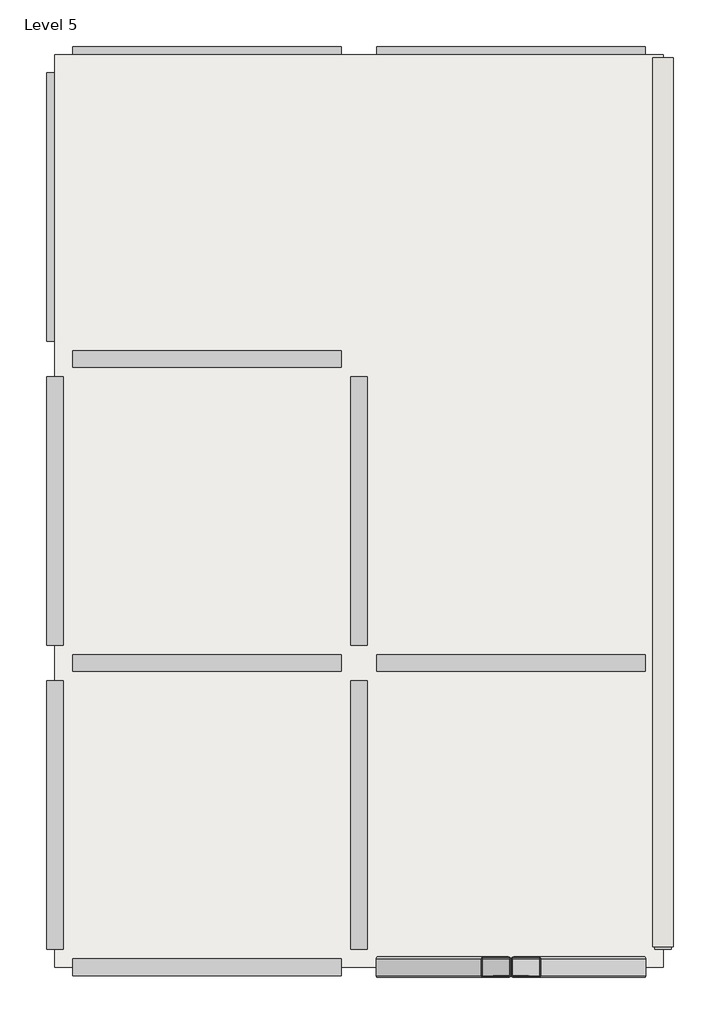
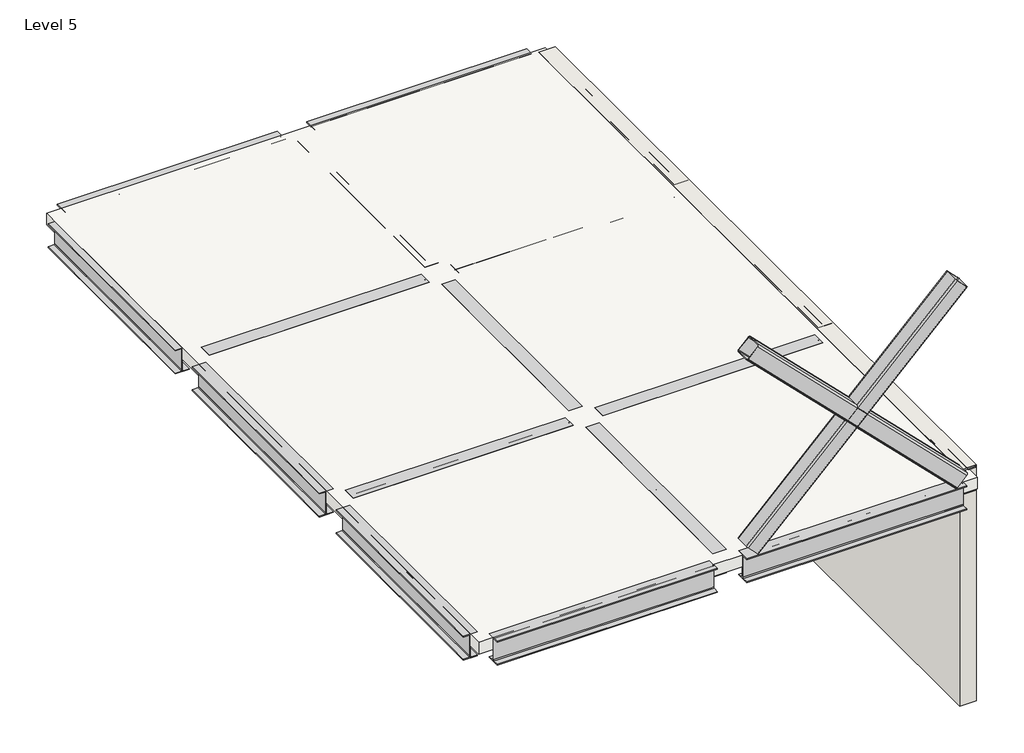
# One storey: 17 beams, 2 members, 1 slab, 1 wall.
"""IFC4 building model written with IfcOpenShell, lengths in millimetres."""

from ifc_helpers import new_model, si_unit, frame, origin, place, context, project, spatial, polyline, outline, extrude, transform, mapped, element, save
from components import ub_universal_beams_ub305x165x40_60ab2ee1, m_hss_square_hss203_2x203_2x9_5_07d005dd

model = new_model("IFC4")

# Units and contexts
model_context = context("Model", 3, world=origin())
ifc_project = project(units=[si_unit("LENGTHUNIT", "METRE", prefix="MILLI")], contexts=[model_context])

# Site, building, storey
site = spatial("IfcSite", under=ifc_project)
building = spatial("IfcBuilding", under=site)
storey = spatial("IfcBuildingStorey", under=building, Name="Level 5", Elevation=12000.0)

# Beams
placement = place(None, origin())
ub_universal_beams_ub305x165x40_shape = ub_universal_beams_ub305x165x40_60ab2ee1(model_context)
element("IfcBeam", 1, ObjectType="UB-Universal Beams : UB305x165x40", at=placement, inside=storey, context=model_context, shape_type="MappedRepresentation", body=[
    mapped(ub_universal_beams_ub305x165x40_shape, transform((18435.1404262, -6314.7314166, 11848.3), x_axis=(-1.0, 0.0, 0.0), y_axis=(0.0, -1.0, 0.0), z_axis=(0.0, 0.0, 1.0))),
])
element("IfcBeam", 2, ObjectType="UB-Universal Beams : UB305x165x40", at=placement, inside=storey, context=model_context, shape_type="MappedRepresentation", body=[
    mapped(ub_universal_beams_ub305x165x40_shape, transform((15435.1404262, -6314.7314166, 11848.3), x_axis=(-1.0, 0.0, 0.0), y_axis=(0.0, -1.0, 0.0), z_axis=(0.0, 0.0, 1.0))),
])
element("IfcBeam", 3, ObjectType="UB-Universal Beams : UB305x165x40", at=placement, inside=storey, context=model_context, shape_type="MappedRepresentation", body=[
    mapped(ub_universal_beams_ub305x165x40_shape, transform((13935.1404262, -4814.7314166, 11848.3), x_axis=(0.0, 1.0, 0.0), y_axis=(-1.0, 0.0, 0.0), z_axis=(0.0, 0.0, 1.0))),
])
element("IfcBeam", 4, ObjectType="UB-Universal Beams : UB305x165x40", at=placement, inside=storey, context=model_context, shape_type="MappedRepresentation", body=[
    mapped(ub_universal_beams_ub305x165x40_shape, transform((13935.1404262, -1814.7314166, 11848.3), x_axis=(0.0, 1.0, 0.0), y_axis=(-1.0, 0.0, 0.0), z_axis=(0.0, 0.0, 1.0))),
])
element("IfcBeam", 5, ObjectType="UB-Universal Beams : UB305x165x40", at=placement, inside=storey, context=model_context, shape_type="MappedRepresentation", body=[
    mapped(ub_universal_beams_ub305x165x40_shape, transform((13935.1404262, 1185.2685834, 11848.3), x_axis=(0.0, 1.0, 0.0), y_axis=(-1.0, 0.0, 0.0), z_axis=(0.0, 0.0, 1.0))),
])
element("IfcBeam", 6, ObjectType="UB-Universal Beams : UB305x165x40", at=placement, inside=storey, context=model_context, shape_type="MappedRepresentation", body=[
    mapped(ub_universal_beams_ub305x165x40_shape, transform((18435.1404262, -3314.7314166, 11848.3), x_axis=(-1.0, 0.0, 0.0), y_axis=(0.0, -1.0, 0.0), z_axis=(0.0, 0.0, 1.0))),
])
element("IfcBeam", 7, ObjectType="UB-Universal Beams : UB305x165x40", at=placement, inside=storey, context=model_context, shape_type="MappedRepresentation", body=[
    mapped(ub_universal_beams_ub305x165x40_shape, transform((15435.1404262, -3314.7314166, 11848.3), x_axis=(-1.0, 0.0, 0.0), y_axis=(0.0, -1.0, 0.0), z_axis=(0.0, 0.0, 1.0))),
])
element("IfcBeam", 8, ObjectType="UB-Universal Beams : UB305x165x40", at=placement, inside=storey, context=model_context, shape_type="MappedRepresentation", body=[
    mapped(ub_universal_beams_ub305x165x40_shape, transform((18435.1404262, -314.7314166, 11848.3), x_axis=(-1.0, 0.0, 0.0), y_axis=(0.0, -1.0, 0.0), z_axis=(0.0, 0.0, 1.0))),
])
element("IfcBeam", 9, ObjectType="UB-Universal Beams : UB305x165x40", at=placement, inside=storey, context=model_context, shape_type="MappedRepresentation", body=[
    mapped(ub_universal_beams_ub305x165x40_shape, transform((15435.1404262, -314.7314166, 11848.3), x_axis=(-1.0, 0.0, 0.0), y_axis=(0.0, -1.0, 0.0), z_axis=(0.0, 0.0, 1.0))),
])
element("IfcBeam", 10, ObjectType="UB-Universal Beams : UB305x165x40", at=placement, inside=storey, context=model_context, shape_type="MappedRepresentation", body=[
    mapped(ub_universal_beams_ub305x165x40_shape, transform((18435.1404262, 2685.2685834, 11848.3), x_axis=(-1.0, 0.0, 0.0), y_axis=(0.0, -1.0, 0.0), z_axis=(0.0, 0.0, 1.0))),
])
element("IfcBeam", 11, ObjectType="UB-Universal Beams : UB305x165x40", at=placement, inside=storey, context=model_context, shape_type="MappedRepresentation", body=[
    mapped(ub_universal_beams_ub305x165x40_shape, transform((15435.1404262, 2685.2685834, 11848.3), x_axis=(-1.0, 0.0, 0.0), y_axis=(0.0, -1.0, 0.0), z_axis=(0.0, 0.0, 1.0))),
])
element("IfcBeam", 12, ObjectType="UB-Universal Beams : UB305x165x40", at=placement, inside=storey, context=model_context, shape_type="MappedRepresentation", body=[
    mapped(ub_universal_beams_ub305x165x40_shape, transform((16935.1404262, -4814.7314166, 11848.3), x_axis=(0.0, 1.0, 0.0), y_axis=(-1.0, 0.0, 0.0), z_axis=(0.0, 0.0, 1.0))),
])
element("IfcBeam", 13, ObjectType="UB-Universal Beams : UB305x165x40", at=placement, inside=storey, context=model_context, shape_type="MappedRepresentation", body=[
    mapped(ub_universal_beams_ub305x165x40_shape, transform((16935.1404262, -1814.7314166, 11848.3), x_axis=(0.0, 1.0, 0.0), y_axis=(-1.0, 0.0, 0.0), z_axis=(0.0, 0.0, 1.0))),
])
element("IfcBeam", 14, ObjectType="UB-Universal Beams : UB305x165x40", at=placement, inside=storey, context=model_context, shape_type="MappedRepresentation", body=[
    mapped(ub_universal_beams_ub305x165x40_shape, transform((16935.1404262, 1185.2685834, 11848.3), x_axis=(0.0, 1.0, 0.0), y_axis=(-1.0, 0.0, 0.0), z_axis=(0.0, 0.0, 1.0))),
])
element("IfcBeam", 15, ObjectType="UB-Universal Beams : UB305x165x40", at=placement, inside=storey, context=model_context, shape_type="MappedRepresentation", body=[
    mapped(ub_universal_beams_ub305x165x40_shape, transform((19935.1404262, -1814.7314166, 11848.3), x_axis=(0.0, 1.0, 0.0), y_axis=(-1.0, 0.0, 0.0), z_axis=(0.0, 0.0, 1.0))),
])
element("IfcBeam", 16, ObjectType="UB-Universal Beams : UB305x165x40", at=placement, inside=storey, context=model_context, shape_type="MappedRepresentation", body=[
    mapped(ub_universal_beams_ub305x165x40_shape, transform((19935.1404262, 1185.2685834, 11848.3), x_axis=(0.0, 1.0, 0.0), y_axis=(-1.0, 0.0, 0.0), z_axis=(0.0, 0.0, 1.0))),
])
element("IfcBeam", 17, ObjectType="UB-Universal Beams : beam", at=placement, inside=storey, context=model_context, shape_type="MappedRepresentation", body=[
    mapped(ub_universal_beams_ub305x165x40_shape, transform((19935.1404262, -4814.7314166, 11848.3), x_axis=(0.0, 1.0, 0.0), y_axis=(-1.0, 0.0, 0.0), z_axis=(0.0, 0.0, 1.0))),
])

# Members
m_hss_square_hss203_2x203_2x9_5_shape = m_hss_square_hss203_2x203_2x9_5_07d005dd(model_context)
element("IfcMember", 18, ObjectType="M_HSS Square : HSS203.2X203.2X9.5", at=placement, inside=storey, context=model_context, shape_type="MappedRepresentation", body=[
    mapped(m_hss_square_hss203_2x203_2x9_5_shape, transform((18435.1404262, -6314.7314166, 13348.3), x_axis=(-0.7071067811865478, 0.0, 0.7071067811865476), y_axis=(0.0, -1.0000000000000002, 0.0), z_axis=(0.7071067811865476, 0.0, 0.7071067811865478))),
])
element("IfcMember", 19, ObjectType="M_HSS Square : HSS203.2X203.2X9.5", at=placement, inside=storey, context=model_context, shape_type="MappedRepresentation", body=[
    mapped(m_hss_square_hss203_2x203_2x9_5_shape, transform((18435.1404262, -6314.7314166, 13348.3), x_axis=(-0.7071067811865478, 0.0, -0.7071067811865475), y_axis=(0.0, -1.0000000000000002, 0.0), z_axis=(-0.7071067811865475, 0.0, 0.7071067811865478))),
])

# Slab
element("IfcSlab", 20, ObjectType="150mm Foundation Slab", at=placement, inside=storey, context=model_context, shape_type="SweptSolid", body=[
    extrude(outline(polyline([(13935.1404262, -6314.7314166), (13935.1404262, 2685.2685834), (19935.1404262, 2685.2685834), (19935.1404262, -6314.7314166), (13935.1404262, -6314.7314166)])), frame((0.0, 0.0, 11850.0), z_axis=(0.0, 0.0, 1.0), x_axis=(1.0, 0.0, 0.0)), (0.0, 0.0, 1.0), 150.0),
])

# Wall
element("IfcWall", 21, ObjectType="Generic - 200mm", at=placement, inside=storey, context=model_context, shape_type="SweptSolid", body=[
    extrude(outline(polyline([(19835.1404262, -6114.7314166), (19835.1404262, 2655.9792615), (20035.1404262, 2655.9792615), (20035.1404262, -6114.7314166), (19835.1404262, -6114.7314166)])), frame((0.0, 0.0, 9000.0), z_axis=(0.0, 0.0, 1.0), x_axis=(1.0, 0.0, 0.0)), (0.0, 0.0, 1.0), 3000.0),
])

save(model, "model.ifc")

# Revit data of these elements
# Type "UB-Universal Beams : UB305x165x40"
#   Section Name Key = "UB305X165X40"
#   Width = 16.5 cm
#   Web Thickness = 0.6 cm
#   Web Fillet = 0.89 cm
#   Warping Constant = 164000.0 cm⁶
#   Torsional Moment of Inertia = 14.70 cm⁴
#   Section Area = 51.3 cm²
#   Plastic Modulus weak axis = 142.0 cm³
#   Plastic Modulus strong axis = 623.0 cm³
#   Nominal Weight = 40.2999 kgf/m
#   Moment of Inertia weak axis = 764.00 cm⁴
#   Moment of Inertia strong axis = 8503.00 cm⁴
#   Height = 30.34 cm
#   Flange Thickness = 1.02 cm
#   Elastic Modulus weak axis = 92.6 cm³
#   Elastic Modulus strong axis = 560.0 cm³
#   Centroid Vertical = 15.17 cm
#   Centroid Horizontal = 8.25 cm
#   Bolt Spacing = 9.0 cm
#   Length [instance default] = 1.5 m
#   Structural Material [instance default] = Metal - Steel 43-275
#   Type Comments = ""
#   Assembly Code = ""
# Type "UB-Universal Beams : beam"
#   Section Name Key = "UB305X165X40"
#   Width = 16.5 cm
#   Web Thickness = 0.6 cm
#   Web Fillet = 0.89 cm
#   Warping Constant = 164000.0 cm⁶
#   Torsional Moment of Inertia = 14.70 cm⁴
#   Section Area = 51.3 cm²
#   Plastic Modulus weak axis = 142.0 cm³
#   Plastic Modulus strong axis = 623.0 cm³
#   Nominal Weight = 40.2999 kgf/m
#   Moment of Inertia weak axis = 764.00 cm⁴
#   Moment of Inertia strong axis = 8503.00 cm⁴
#   Height = 30.34 cm
#   Flange Thickness = 1.02 cm
#   Elastic Modulus weak axis = 92.6 cm³
#   Elastic Modulus strong axis = 560.0 cm³
#   Centroid Vertical = 15.17 cm
#   Centroid Horizontal = 8.25 cm
#   Bolt Spacing = 9.0 cm
#   Length [instance default] = 1.5 m
#   Structural Material [instance default] = Metal - Steel 43-275
#   Type Comments = ""
#   Assembly Code = ""
# Type "M_HSS Square : HSS203.2X203.2X9.5"
#   Section Name Key = "HSS 8X8X3/8"
#   Width = 20.3 cm
#   Wall Nominal Thickness = 0.953 cm
#   Wall Design Thickness = 0.886 cm
#   Torsional Moment of Inertia = 6660.00 cm⁴
#   Torsional Modulus = 10930171.7 cm³
#   Section Area = 67.1 cm²
#   Plastic Modulus weak axis = 482.0 cm³
#   Plastic Modulus strong axis = 482.0 cm³
#   Outer Fillet = 1.906 cm
#   Nominal Weight = 55.9998 kgf/m
#   Moment of Inertia weak axis = 4160.00 cm⁴
#   Moment of Inertia strong axis = 4160.00 cm⁴
#   Length [instance default] = 1.524 m
#   Inner Fillet = 0.953 cm
#   Height = 20.3 cm
#   Elastic Modulus weak axis = 408.0 cm³
#   Elastic Modulus strong axis = 408.0 cm³
#   Centroid Vertical = 10.15 cm
#   Centroid Horizontal = 10.15 cm
#   Structural Material [instance default] = Steel, 45-345
# Type "150mm Foundation Slab"
#   Layers, outside or top first: 0.15 m "Concrete, Cast-in-Place gray" (function 1)
# Type "Generic - 200mm"
#   Layers, outside or top first: 0.2 m no material (function 1)
# Elements 1, 2, 3, 4, 5, 6, 7, 8, 9, 10, 11, 12, 13, 14, 15, 16 (IfcBeam, "UB-Universal Beams : UB305x165x40")
#   Structural Material = Metal - Steel 43-275
#   Phase Created = New Construction
#   Materials on its faces: "Metal - Steel 43-275"
# Element 17 (IfcBeam, "UB-Universal Beams : beam")
#   Structural Material = Metal - Steel 43-275
#   Phase Created = New Construction
#   Materials on its faces: "Metal - Steel 43-275"
# Elements 18, 19 (IfcMember, "M_HSS Square : HSS203.2X203.2X9.5")
#   Comments = ""
#   Structural Material = Metal - Steel 43-275
#   Phase Created = New Construction
#   Materials on its faces: "Metal - Steel 43-275"
# Element 20 (IfcSlab, "150mm Foundation Slab")
#   built-in parameter 1001955 = 3.14159 (stored number, unit not read)
#   Height Offset From Level = 0 m
#   built-in parameter 1001954 = 1
#   Phase Created = New Construction
#   Materials on its faces: "Concrete, Cast-in-Place gray"
# Element 21 (IfcWall, "Generic - 200mm")
#   Comments = ""
#   built-in parameter 1001111 = -3 m
#   Top Offset = 0 m
#   Base Offset = -3 m
#   wall height = 3 m
#   Phase Created = New Construction
#   Base Constraint = Level 5
#   Top Constraint = Level 5
#   Materials on its faces: "Default Wall"
# Materials
#   "Metal - Steel 43-275": class "Metal", colour RGB 247 247 247, transparency 0, Cost = 0
#   "Steel, 45-345": class "Metal", colour RGB 247 247 247, transparency 0, Description = "Steel 345 MPa", Cost = 0
#   "Concrete, Cast-in-Place gray": class "Concrete", colour RGB 192 192 192, transparency 0, Description = "Cast-in-place concrete", Cost = 0
#   "Default Wall": colour RGB 128 128 128, transparency 0, Cost = 0
